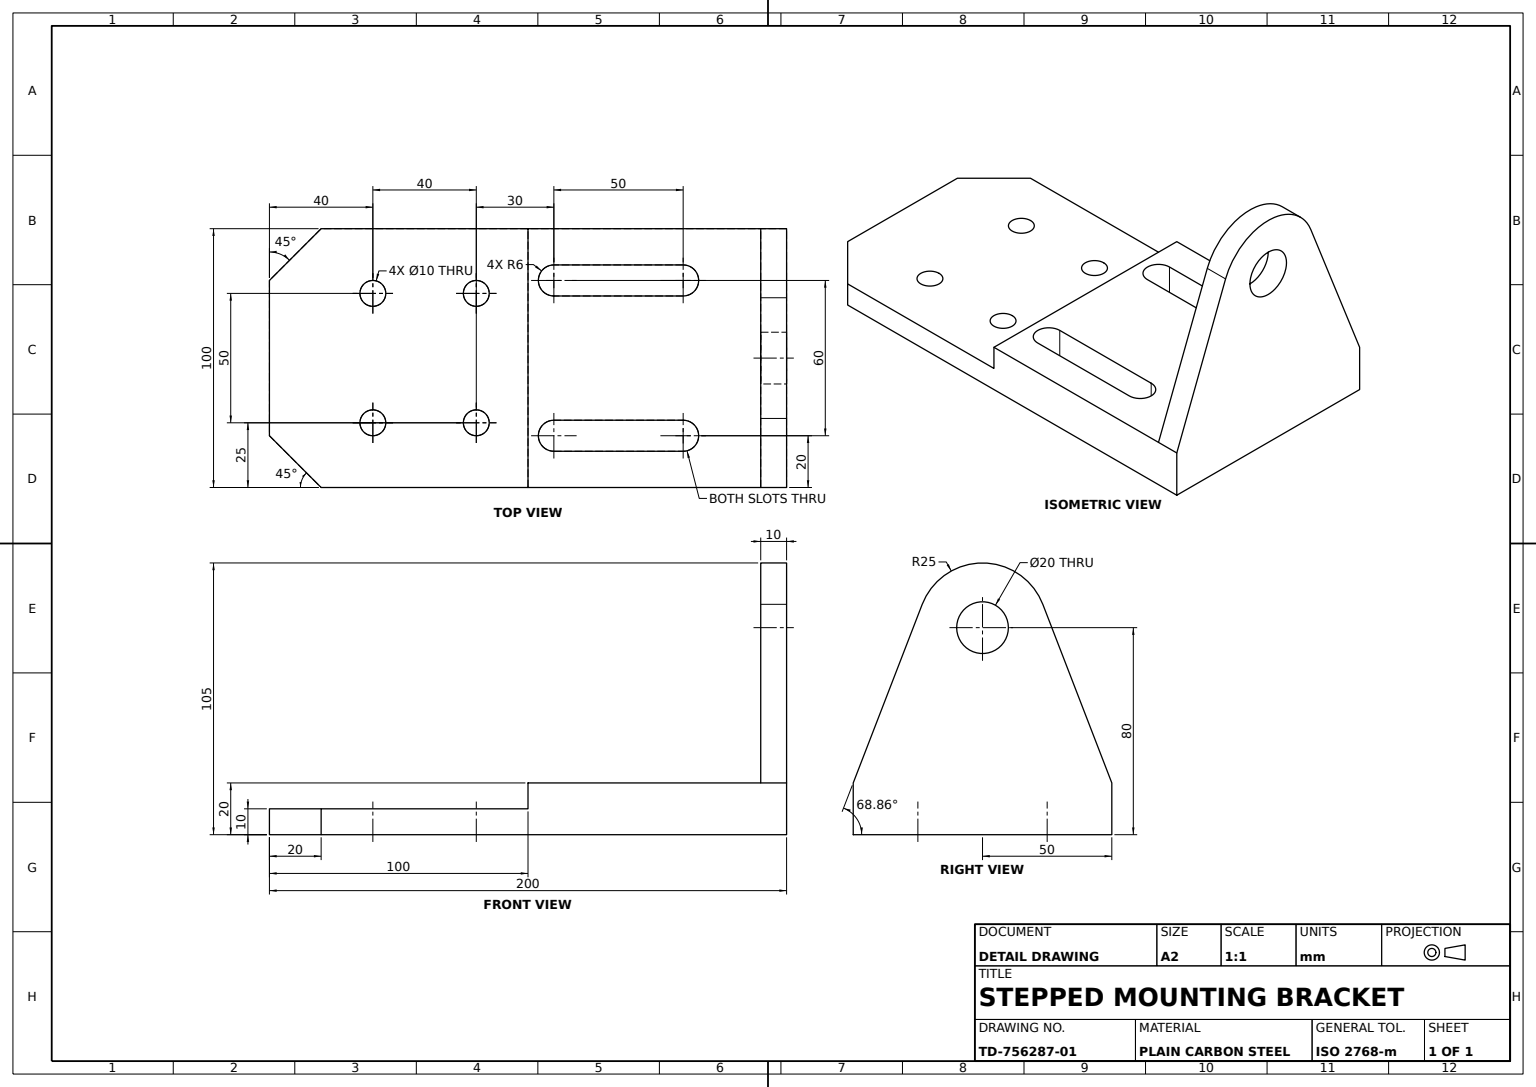
from build123d import *

# Parameters (mm, degrees)
BASE_PLATE_SKETCH_W             = 100
BASE_PLATE_SKETCH_H             = 20
BASE_PLATE_DEPTH                = 100
MOUNTING_FLANGE_SKETCH_W        = 100
MOUNTING_FLANGE_SKETCH_H        = 100
MOUNTING_FLANGE_DEPTH           = 10
FLANGE_CORNER_CHAMFER_20MM_SIZE = 20
LUG_PROFILE_SKETCH_R            = 10
UPRIGHT_LUG_DEPTH               = 10
ADJUSTMENT_SLOTS_2X_DEPTH       = 166
MOUNTING_HOLES_SKETCH_R         = 5
FLANGE_MOUNTING_HOLES_DEPTH     = 10


with BuildPart() as part:
    # Base Plate Sketch → Base Plate (new body)
    with BuildSketch(Plane.XY):
        with Locations((50, 10)):
            Rectangle(BASE_PLATE_SKETCH_W, BASE_PLATE_SKETCH_H)
    extrude(amount=BASE_PLATE_DEPTH)

    # Mounting Flange Sketch → Mounting Flange (add)
    with BuildSketch(Plane(origin=(0, 0, 0), x_dir=(1, 0, 0), z_dir=(0, 1, 0))):
        with Locations((-50, -50)):
            Rectangle(MOUNTING_FLANGE_SKETCH_W, MOUNTING_FLANGE_SKETCH_H)
    extrude(amount=MOUNTING_FLANGE_DEPTH)

    # Flange Corner Chamfer 20mm
    flange_corner_chamfer_20mm_edges = [part.edges().sort_by_distance(p)[0] for p in [
        (-100, 5, 0),
        (-100, 5, 100),
    ]]
    chamfer(flange_corner_chamfer_20mm_edges, length=FLANGE_CORNER_CHAMFER_20MM_SIZE)

    # Lug Profile Sketch → Upright Lug (add)
    with BuildSketch(Plane(origin=(100, 0, 0), x_dir=(0, 0, -1), z_dir=(1, 0, 0))):
        with BuildLine():
            Line((-100, 20), (-73.318010558, 89.015008798))
            ThreePointArc((-73.318010558, 89.015008798), (-50, 105), (-26.681989442, 89.015008798))
            Line((-26.681989442, 89.015008798), (0, 20))
            Line((0, 20), (-100, 20))
        make_face()
        with Locations((-50, 80)):
            Circle(LUG_PROFILE_SKETCH_R, mode=Mode.SUBTRACT)
    extrude(amount=-UPRIGHT_LUG_DEPTH)

    # Adjustment Slots Sketch → Adjustment Slots 2x (cut, through all)
    with BuildSketch(Plane(origin=(0, 20, 0), x_dir=(1, 0, 0), z_dir=(0, 1, 0))):
        with BuildLine():
            Line((10, -14), (60, -14))
            ThreePointArc((60, -14), (66, -20), (60, -26))
            Line((60, -26), (10, -26))
            ThreePointArc((10, -26), (4, -20), (10, -14))
        make_face()
        with BuildLine():
            Line((60, -86), (10, -86))
            ThreePointArc((10, -86), (4, -80), (10, -74))
            Line((10, -74), (60, -74))
            ThreePointArc((60, -74), (66, -80), (60, -86))
        make_face()
    extrude(amount=-ADJUSTMENT_SLOTS_2X_DEPTH, mode=Mode.SUBTRACT)

    # Mounting Holes Sketch → Flange Mounting Holes (cut)
    with BuildSketch(Plane(origin=(0, 10, 0), x_dir=(1, 0, 0), z_dir=(0, 1, 0))):
        with Locations(Location((-20, -25, 0), (0, 0, 270))):
            Circle(MOUNTING_HOLES_SKETCH_R)
        with Locations(Location((-60, -25, 0), (0, 0, 270))):
            Circle(MOUNTING_HOLES_SKETCH_R)
        with Locations(Location((-20, -75, 0), (0, 0, 270))):
            Circle(MOUNTING_HOLES_SKETCH_R)
        with Locations(Location((-60, -75, 0), (0, 0, 270))):
            Circle(MOUNTING_HOLES_SKETCH_R)
    extrude(amount=-FLANGE_MOUNTING_HOLES_DEPTH, mode=Mode.SUBTRACT)


solid = part.part
